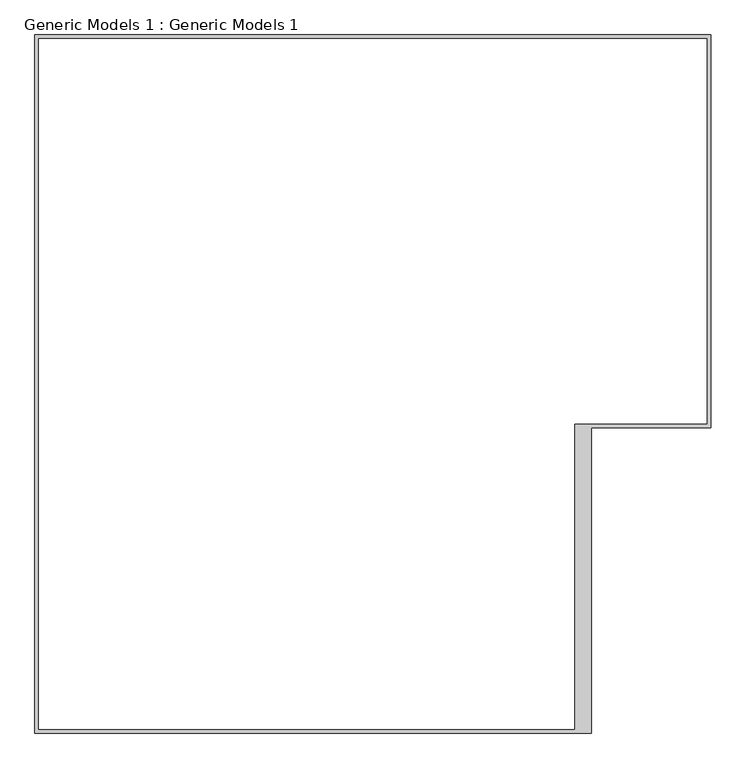
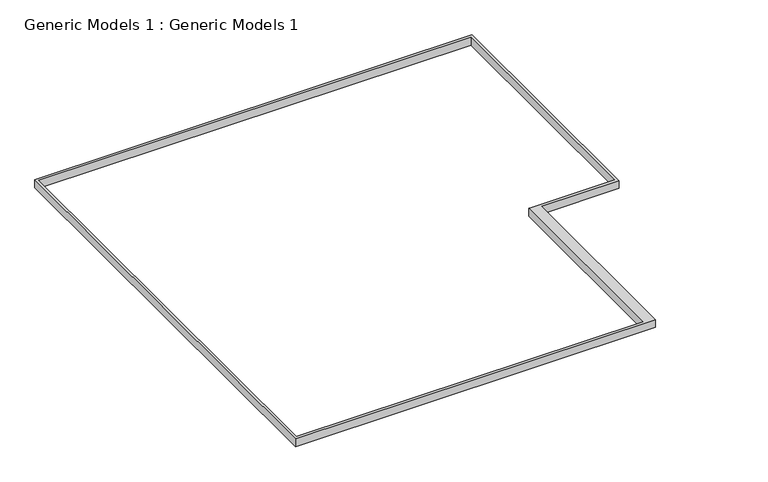
"""IFC4 building model written with IfcOpenShell, lengths in millimetres: proxy geometry, Generic Models 1 : Generic Models 1."""

from ifc_helpers import new_model, si_unit, frame, origin, place, context, project, spatial, polyline, outline, extrude, source, transform, mapped, element, save


def generic_models_1_generic_models_1_9ce5a9d9(model_context):
    return source(origin(), model_context, "Body", "SweptSolid", [
        extrude(outline(polyline([(-8561.3723897, -5347.4557833), (-8561.3723897, -1807.0124134), (-5131.5238298, -1807.0124134), (-5131.5238298, -3798.5041511), (-5738.2504128, -3798.5041511), (-5738.2504128, -5347.4557833), (-8561.3723897, -5347.4557833)]), holes=[polyline([(-8541.3302022, -5327.4135958), (-5823.543721, -5327.4135958), (-5823.543721, -3778.4619636), (-5151.5660173, -3778.4619636), (-5151.5660173, -1827.0546009), (-8541.3302022, -1827.0546009), (-8541.3302022, -5327.4135958)])]), frame((0.0, 0.0, 2568.8778018), z_axis=(0.0, 0.0, 1.0), x_axis=(1.0, 0.0, 0.0)), (0.0, 0.0, 1.0), 64.9464778),
    ])


if __name__ == "__main__":
    model = new_model("IFC4")
    model_context = context("Model", 3, world=origin())
    ifc_project = project(units=[si_unit("LENGTHUNIT", "METRE", prefix="MILLI")], contexts=[model_context])
    site = spatial("IfcSite", under=ifc_project)
    building = spatial("IfcBuilding", under=site)
    placement = place(None, origin())
    generic_models_1_generic_models_1_shape = generic_models_1_generic_models_1_9ce5a9d9(model_context)
    element("IfcBuildingElementProxy", 1, Name="Generic Models 1 : Generic Models 1", ObjectType="Generic Models 1 : Generic Models 1", at=placement, inside=building, context=model_context, shape_type="MappedRepresentation", body=[
        mapped(generic_models_1_generic_models_1_shape, transform((0.0, 0.0, 0.0), x_axis=(1.0, 0.0, 0.0), y_axis=(0.0, 1.0, 0.0), z_axis=(0.0, 0.0, 1.0))),
    ])
    save(model, "model.ifc")

# Revit data of these elements
# Element 1 (IfcBuildingElementProxy, "Generic Models 1 : Generic Models 1")
#   Materials on its faces: "SAN PLASTIC"
# Materials
#   "SAN PLASTIC": class "Generic", colour RGB 120 120 120, transparency 0, Cost = 0
